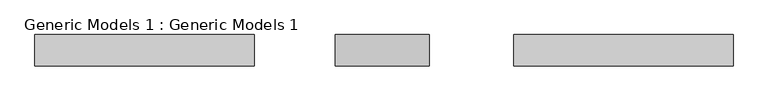
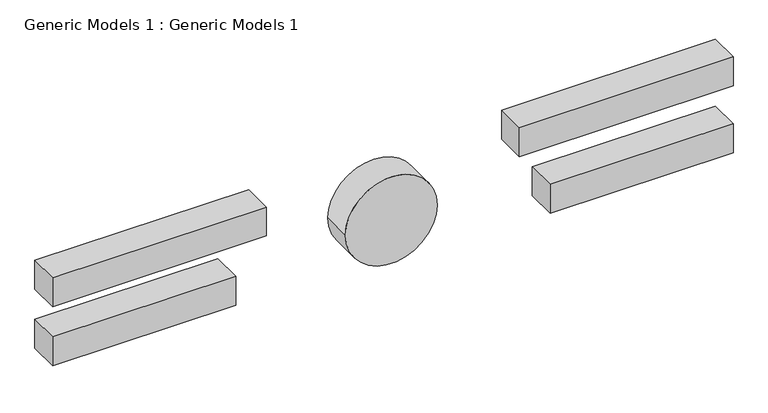
"""IFC4 building model written with IfcOpenShell, lengths in millimetres: proxy geometry, Generic Models 1 : Generic Models 1."""

from ifc_helpers import new_model, si_unit, point, frame, frame_2d, origin, place, context, project, spatial, polyline, circle_curve, trimmed, segment, composite_curve, outline, extrude, source, transform, mapped, element, save


def generic_models_1_generic_models_1_124607eb(model_context):
    return source(origin(), model_context, "Body", "SweptSolid", [
        extrude(outline(composite_curve([segment(trimmed(circle_curve(frame_2d((16762.061959, -1312.6050488)), 457.2), [point((16762.061959, -1769.8050488))], [point((16762.061959, -855.4050488))], False, "CARTESIAN"), True, "CONTINUOUS"), segment(trimmed(circle_curve(frame_2d((16762.061959, -1312.6050488)), 457.2), [point((16762.061959, -855.4050488))], [point((16762.061959, -1769.8050488))], False, "CARTESIAN"), True, "CONTINUOUS")], self_intersect=False)), frame((0.0, -5458.1109248, 0.0), z_axis=(0.0, 1.0, 0.0), x_axis=(0.0, 0.0, 1.0)), (0.0, 0.0, 1.0), 304.8),
        extrude(outline(polyline([(2102.2056353, -5458.1109248), (-31.3943647, -5458.1109248), (-31.3943647, -5153.3109248), (2102.2056353, -5153.3109248), (2102.2056353, -5458.1109248)])), frame((0.0, 0.0, 16984.975557), z_axis=(0.0, 0.0, 1.0), x_axis=(1.0, 0.0, 0.0)), (0.0, 0.0, 1.0), 304.8),
        extrude(outline(polyline([(2102.2056353, -5458.1109248), (273.4056353, -5458.1109248), (273.4056353, -5153.3109248), (2102.2056353, -5153.3109248), (2102.2056353, -5458.1109248)])), frame((0.0, 0.0, 16279.0247452), z_axis=(0.0, 0.0, 1.0), x_axis=(1.0, 0.0, 0.0)), (0.0, 0.0, 1.0), 304.8),
        extrude(outline(polyline([(-2562.4839679, -5458.1109248), (-4696.0839679, -5458.1109248), (-4696.0839679, -5153.3109248), (-2562.4839679, -5153.3109248), (-2562.4839679, -5458.1109248)])), frame((0.0, 0.0, 17033.3417411), z_axis=(0.0, 0.0, 1.0), x_axis=(1.0, 0.0, 0.0)), (0.0, 0.0, 1.0), 304.8),
        extrude(outline(polyline([(-2867.2839679, -5458.1109248), (-4696.0839679, -5458.1109248), (-4696.0839679, -5153.3109248), (-2867.2839679, -5153.3109248), (-2867.2839679, -5458.1109248)])), frame((0.0, 0.0, 16409.222856), z_axis=(0.0, 0.0, 1.0), x_axis=(1.0, 0.0, 0.0)), (0.0, 0.0, 1.0), 304.8),
    ])


if __name__ == "__main__":
    model = new_model("IFC4")
    model_context = context("Model", 3, world=origin())
    ifc_project = project(units=[si_unit("LENGTHUNIT", "METRE", prefix="MILLI")], contexts=[model_context])
    site = spatial("IfcSite", under=ifc_project)
    building = spatial("IfcBuilding", under=site)
    placement = place(None, origin())
    generic_models_1_generic_models_1_shape = generic_models_1_generic_models_1_124607eb(model_context)
    element("IfcBuildingElementProxy", 1, Name="Generic Models 1 : Generic Models 1", ObjectType="Generic Models 1 : Generic Models 1", at=placement, inside=building, context=model_context, shape_type="MappedRepresentation", body=[
        mapped(generic_models_1_generic_models_1_shape, transform((0.0, 0.0, 0.0), x_axis=(1.0, 0.0, 0.0), y_axis=(0.0, 1.0, 0.0), z_axis=(0.0, 0.0, 1.0))),
    ])
    save(model, "model.ifc")

# Revit data of these elements
# Element 1 (IfcBuildingElementProxy, "Generic Models 1 : Generic Models 1")
#   Materials on its faces: "Default Mass Exterior Wall", "Parking Stripe"
# Materials
#   "Default Mass Exterior Wall": class "Generic", colour RGB 133 178 44, transparency 0.2, Cost = 0
#   "Parking Stripe": class "Paint", colour RGB 250 250 91, transparency 0, Cost = 0
